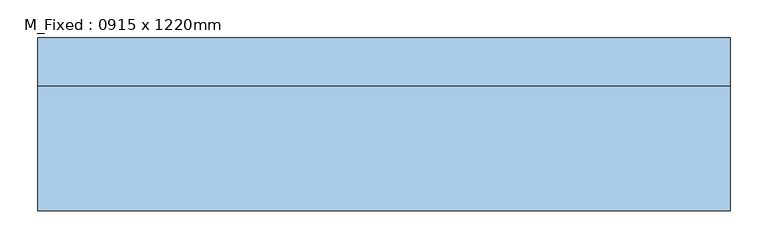
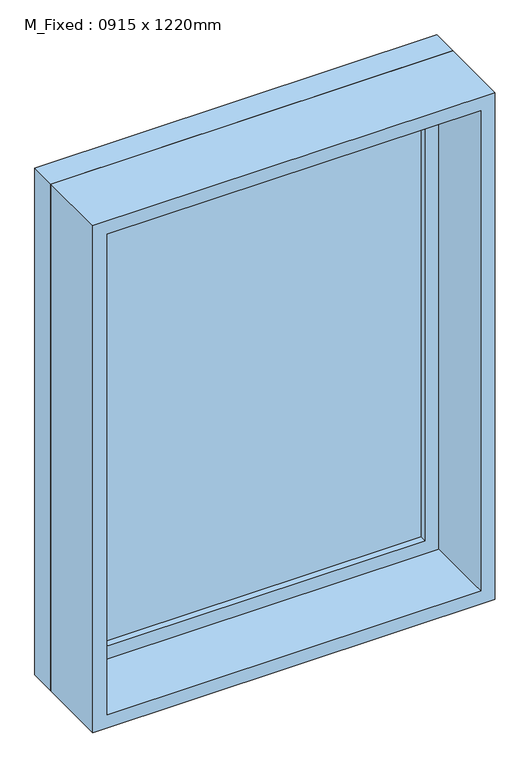
"""IFC4 building model written with IfcOpenShell, lengths in millimetres: window geometry, M_Fixed : 0915 x 1220mm."""

from ifc_helpers import new_model, si_unit, frame, origin, place, context, project, spatial, polyline, outline, extrude, source, transform, mapped, element, save


def m_fixed_0915_x_1220mm_b7e646b7(model_context):
    return source(origin(), model_context, "Body", "SweptSolid", [
        extrude(outline(polyline([(-394.5, 92.3), (394.5, 92.3), (394.5, 80.3), (-394.5, 80.3), (-394.5, 92.3)])), frame((0.0, 0.0, 978.0), z_axis=(0.0, 0.0, 1.0), x_axis=(1.0, 0.0, 0.0)), (0.0, 0.0, 1.0), 1094.0),
        extrude(outline(polyline([(2116.0, -438.5), (934.0, -438.5), (934.0, 438.5), (2116.0, 438.5), (2116.0, -438.5)]), holes=[polyline([(2072.0, -394.5), (2072.0, 394.5), (978.0, 394.5), (978.0, -394.5), (2072.0, -394.5)])]), frame((0.0, 64.3, 0.0), z_axis=(0.0, 1.0, 0.0), x_axis=(0.0, 0.0, 1.0)), (0.0, 0.0, 1.0), 44.0),
        extrude(outline(polyline([(2135.0, -457.5), (915.0, -457.5), (915.0, 457.5), (2135.0, 457.5), (2135.0, -457.5)]), holes=[polyline([(2116.0, -438.5), (2116.0, 438.5), (934.0, 438.5), (934.0, -438.5), (2116.0, -438.5)])]), frame((0.0, 64.3, 0.0), z_axis=(0.0, 1.0, 0.0), x_axis=(0.0, 0.0, 1.0)), (0.0, 0.0, 1.0), 63.0),
        extrude(outline(polyline([(2135.0, -457.5), (915.0, -457.5), (915.0, 457.5), (2135.0, 457.5), (2135.0, -457.5)]), holes=[polyline([(2103.0, -425.5), (2103.0, 425.5), (947.0, 425.5), (947.0, -425.5), (2103.0, -425.5)])]), frame((0.0, -101.3, 0.0), z_axis=(0.0, 1.0, 0.0), x_axis=(0.0, 0.0, 1.0)), (0.0, 0.0, 1.0), 165.6),
    ])


if __name__ == "__main__":
    model = new_model("IFC4")
    model_context = context("Model", 3, world=origin())
    ifc_project = project(units=[si_unit("LENGTHUNIT", "METRE", prefix="MILLI")], contexts=[model_context])
    site = spatial("IfcSite", under=ifc_project)
    building = spatial("IfcBuilding", under=site)
    placement = place(None, origin())
    m_fixed_0915_x_1220mm_shape = m_fixed_0915_x_1220mm_b7e646b7(model_context)
    element("IfcWindow", 1, ObjectType="M_Fixed : 0915 x 1220mm", at=placement, inside=building, context=model_context, shape_type="MappedRepresentation", body=[
        mapped(m_fixed_0915_x_1220mm_shape, transform((0.0, 0.0, 0.0), x_axis=(1.0, 0.0, 0.0), y_axis=(0.0, 1.0, 0.0), z_axis=(0.0, 0.0, 1.0))),
    ])
    save(model, "model.ifc")

# Revit data of these elements
# Type "M_Fixed : 0915 x 1220mm"
#   Type Mark = "15"
#   Height = 1220 mm
#   Default Sill Height = 915 mm
#   Width = 915 mm
#   Window Inset = 19 mm
#   Frame Exterior Material = Sash
#   Frame Interior Material = Sash
#   Glass Pane Material = Glass
#   Sash = Sash
#   Wall Closure = (empty or 0)
# Element 1 (IfcWindow, "M_Fixed : 0915 x 1220mm")
#   Materials on its faces: "Sash", "Glass"
# Materials
#   "Sash": class "Wood", colour RGB 136 99 55, transparency 0
#   "Glass": class "Glass", colour RGB 218 227 224, transparency 0.85, Description = "Soda Lime Glass", Cost = 0
